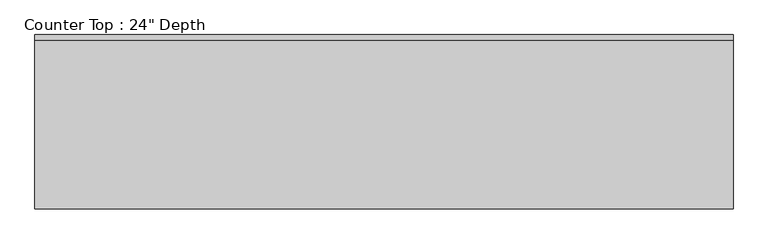
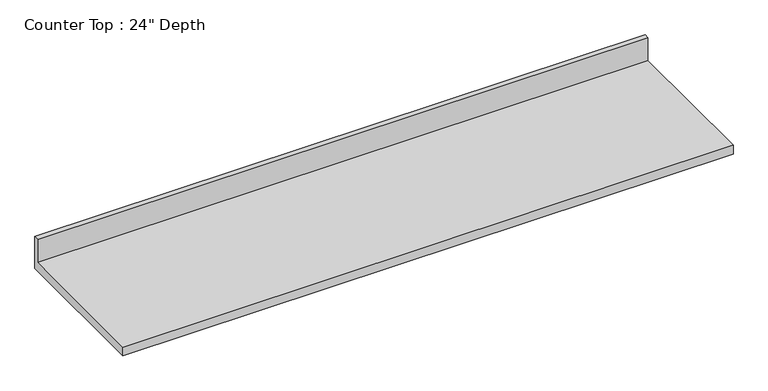
"""IFC4 building model written with IfcOpenShell, lengths in millimetres: furniture geometry."""

from ifc_helpers import new_model, si_unit, frame, origin, place, context, project, spatial, polyline, outline, extrude, source, transform, mapped, element, save


def furniture_c0b19bce(model_context):
    return source(origin(), model_context, "Body", "SweptSolid", [
        extrude(outline(polyline([(0.0, 1016.0), (0.0, 876.3), (-635.0, 876.3), (-635.0, 914.4), (-19.05, 914.4), (-19.05, 1016.0), (0.0, 1016.0)])), frame((-1200.4622951, 0.0, 0.0), z_axis=(1.0, 0.0, 0.0), x_axis=(0.0, 1.0, 0.0)), (0.0, 0.0, 1.0), 2540.0),
    ])


if __name__ == "__main__":
    model = new_model("IFC4")
    model_context = context("Model", 3, world=origin())
    ifc_project = project(units=[si_unit("LENGTHUNIT", "METRE", prefix="MILLI")], contexts=[model_context])
    site = spatial("IfcSite", under=ifc_project)
    building = spatial("IfcBuilding", under=site)
    placement = place(None, origin())
    furniture_shape = furniture_c0b19bce(model_context)
    element("IfcFurniture", 1, ObjectType="Counter Top : 24\" Depth", at=placement, inside=building, context=model_context, shape_type="MappedRepresentation", body=[
        mapped(furniture_shape, transform((0.0, 0.0, 0.0), x_axis=(1.0, 0.0, 0.0), y_axis=(0.0, 1.0, 0.0), z_axis=(0.0, 0.0, 1.0))),
    ])
    save(model, "model.ifc")

# Revit data of these elements
# Type "Counter Top : 24\" Depth"
#   Assembly Code = "C1030400"
#   Counter Thickness = 0' - 1 1/2"
#   Depth = 2' - 1"
#   Height = 3' - 0"
#   Length [instance default] = 8' - 0"
#   Counter Top Material = none
#   Default Elevation = 0
# Element 1 (IfcFurniture, "Counter Top : 24\" Depth")
#   Length = 8' - 4"
#   Materials on its faces: "Counter Top"
# Materials
#   "Counter Top": class "Wood", colour RGB 226 177 128, transparency 0
